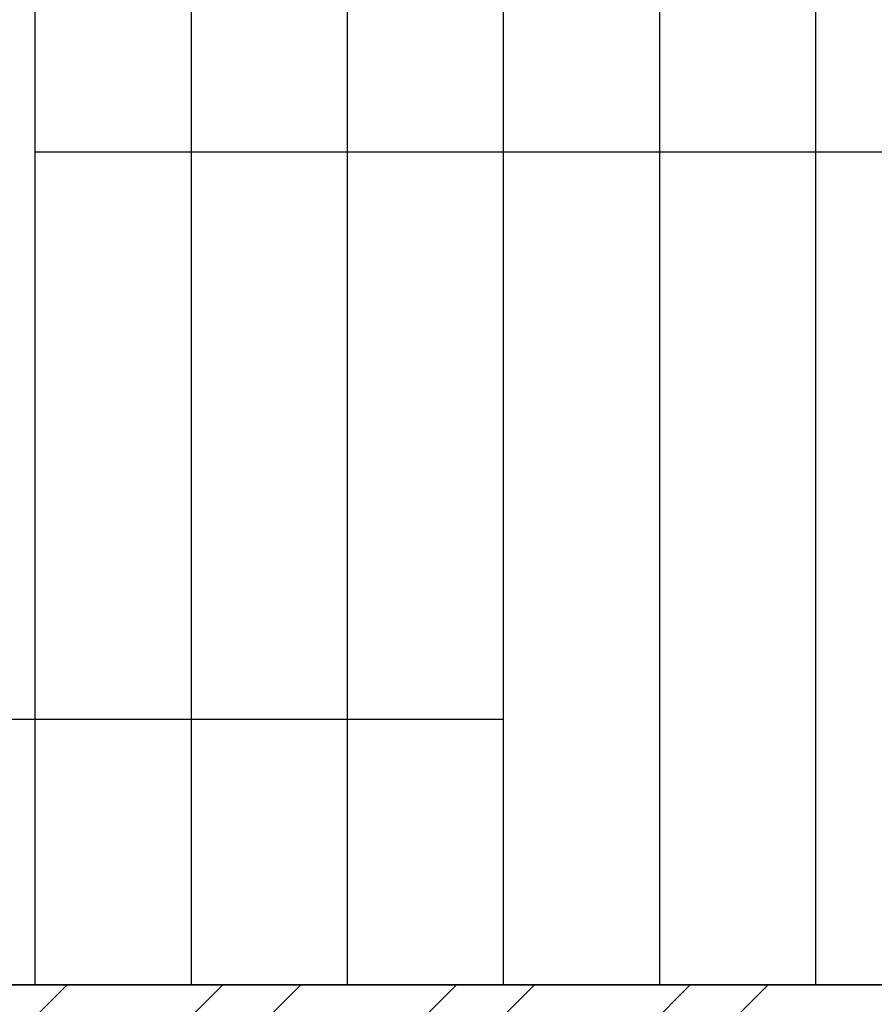
# Model space of a CAD drawing. Units: inches. Extents: x 1962 to 2771, y 1245 to 2660.
# Tile 34 of 114: x 2110 to 2159, y 1932 to 1989. Entities that reach past the tile are written whole.
import ezdxf

# ---------------------------------------------------------------- set-up
doc = ezdxf.new("R2010")
doc.units = ezdxf.units.IN
for name, color, linetype, lineweight in [('A-FLOR-STRS', 7, 'Continuous', 25), ('A-WALL', 7, 'Continuous', 35), ('A-WALL-PATT', 252, 'Continuous', 13)]:
    doc.layers.add(name, color=color, linetype=linetype, lineweight=lineweight)

msp = doc.modelspace()

# ---------------------------------------------------------------- hatches: boundary and pattern name
at = {"layer": 'A-WALL-PATT'}
h = msp.add_hatch(dxfattribs=at)
h.set_pattern_fill('ANSI32', color=256)
h.paths.add_polyline_path([(2090.8074, 2467.3437), (2141.6481, 2467.3437), (2141.6481, 2469.5937), (2141.6481, 2471.8437), (2086.3074, 2471.8437), (2086.3074, 2422.5333), (2090.8074, 2422.5333)])
h.paths.add_polyline_path([(2282.7664, 2471.8437), (2204.8982, 2471.8437), (2204.8982, 2467.3437), (2234.8074, 2467.3437), (2234.8074, 2311.3437), (2228.7492, 2311.3437), (2228.7492, 2306.8437), (2234.8074, 2306.8437), (2331.9227, 2306.8437), (2331.9227, 2309.0937), (2331.9227, 2311.3437), (2239.3074, 2311.3437), (2239.3074, 2467.3437), (2282.7664, 2467.3437), (2282.7664, 2469.5937)])
h.paths.add_polyline_path([(2471.4531, 2519.8437), (2552.011, 2519.8437), (2564.3996, 2519.8437), (2564.3996, 2511.1389), (2568.8996, 2511.1389), (2568.8996, 2524.3437), (2466.9531, 2524.3437), (2466.9531, 2471.8437), (2450.0749, 2471.8437), (2446.4672, 2471.8437), (2446.4672, 2467.3437), (2450.0749, 2467.3437), (2475.9988, 2467.3437), (2475.9988, 2469.5937), (2475.9988, 2471.8437), (2471.4531, 2471.8437)])
h.paths.add_polyline_path([(2575.2231, 2469.5937), (2575.2231, 2471.8437), (2568.8996, 2471.8437), (2568.8996, 2487.1389), (2564.3996, 2487.1389), (2564.3996, 2471.8437), (2556.511, 2471.8437), (2499.2904, 2471.8437), (2499.2904, 2467.3437), (2507.8074, 2467.3437), (2507.8074, 2311.3437), (2414.863, 2311.3437), (2414.863, 2306.8437), (2512.3074, 2306.8437), (2517.0114, 2306.8437), (2517.0114, 2309.0937), (2517.0114, 2311.3437), (2512.3074, 2311.3437), (2512.3074, 2467.3437), (2575.2231, 2467.3437)])
h.paths.add_polyline_path([(2660.8074, 2471.8437), (2600.9602, 2471.8437), (2600.9602, 2467.3437), (2656.3074, 2467.3437), (2656.3074, 2432.5704), (2660.8074, 2432.5704)])
h.paths.add_polyline_path([(2660.8074, 2372.5704), (2656.3074, 2372.5704), (2656.3074, 2311.3437), (2600.276, 2311.3437), (2600.276, 2309.0937), (2600.276, 2306.8437), (2656.3074, 2306.8437), (2656.3074, 2296.2593), (2660.8074, 2296.2593)])
h.paths.add_polyline_path([(2572.3074, 2306.8437), (2577.1385, 2306.8437), (2577.1385, 2311.3437), (2551.082, 2311.3437), (2551.082, 2306.8437), (2567.8074, 2306.8437), (2567.8074, 2258.8437), (2540.0574, 2258.8437), (2540.0574, 2256.5937), (2540.0574, 2254.3437), (2567.8074, 2254.3437), (2656.3074, 2254.3437), (2656.3074, 2236.9085), (2660.8074, 2236.9085), (2660.8074, 2272.2593), (2656.3074, 2272.2593), (2656.3074, 2258.8437), (2572.3074, 2258.8437)])
h.paths.add_polyline_path([(2512.3074, 2254.3437), (2518.8716, 2254.3437), (2518.8716, 2256.5937), (2518.8716, 2258.8437), (2507.8074, 2258.8437), (2507.8074, 2177.8437), (2567.8074, 2177.8437), (2567.8074, 2172.9628), (2572.3074, 2172.9628), (2572.3074, 2177.8437), (2656.3074, 2177.8437), (2656.3074, 2166.4846), (2660.8074, 2166.4846), (2660.8074, 2200.9085), (2656.3074, 2200.9085), (2656.3074, 2182.3437), (2512.3074, 2182.3437)])
h.paths.add_polyline_path([(2656.3074, 2129.8437), (2572.3074, 2129.8437), (2572.3074, 2150.3044), (2570.0574, 2150.3044), (2567.8074, 2150.3044), (2567.8074, 2129.8437), (2507.8074, 2129.8437), (2507.8074, 2116.3027), (2510.0574, 2116.3027), (2512.3074, 2116.3027), (2512.3074, 2125.3437), (2567.8074, 2125.3437), (2572.3074, 2125.3437), (2656.3074, 2125.3437)])
h.paths.add_polyline_path([(2090.8074, 2362.5333), (2086.3074, 2362.5333), (2086.3074, 2298.6242), (2090.8074, 2298.6242), (2090.8074, 2306.8437), (2174.8074, 2306.8437), (2174.8074, 2286.4178), (2179.3074, 2286.4178), (2179.3074, 2306.8437), (2192.8641, 2306.8437), (2192.8641, 2309.0937), (2192.8641, 2311.3437), (2090.8074, 2311.3437)])
h.paths.add_polyline_path([(2209.156, 2258.8437), (2179.3074, 2258.8437), (2179.3074, 2263.2236), (2177.0574, 2263.2236), (2174.8074, 2263.2236), (2174.8074, 2258.8437), (2090.8074, 2258.8437), (2090.8074, 2274.6242), (2086.3074, 2274.6242), (2086.3074, 2238.2967), (2088.5574, 2238.2967), (2090.8074, 2238.2967), (2090.8074, 2254.3437), (2209.156, 2254.3437)])
h.paths.add_polyline_path([(2090.8074, 2177.8437), (2234.8074, 2177.8437), (2234.8074, 2173.1428), (2239.3074, 2173.1428), (2239.3074, 2258.8437), (2230.8442, 2258.8437), (2230.8442, 2256.5937), (2230.8442, 2254.3437), (2234.8074, 2254.3437), (2234.8074, 2182.3437), (2090.8074, 2182.3437), (2090.8074, 2202.2967), (2086.3074, 2202.2967), (2086.3074, 2140.0389), (2090.8074, 2140.0389)])
h.paths.add_polyline_path([(2090.8074, 2080.0389), (2086.3074, 2080.0389), (2086.3074, 2033.8437), (2090.8074, 2033.8437)], flags=17)
h.paths.add_polyline_path([(2244.9405, 2033.8437), (2239.3074, 2033.8437), (2239.3074, 2142.0665), (2237.2592, 2142.0665), (2234.8074, 2142.0665), (2234.8074, 2033.8437), (2090.8074, 2033.8437), (2076.5204, 2033.8437), (2072.0204, 2033.8437), (2072.0204, 2000.4493), (2076.5204, 2000.4493), (2076.5204, 2029.3437), (2090.8074, 2029.3437), (2244.9405, 2029.3437), (2244.9405, 2031.5937)])
h.paths.add_polyline_path([(2234.8074, 1933.3437), (2076.5204, 1933.3437), (2076.5204, 1952.4493), (2074.2704, 1952.4493), (2072.0204, 1952.4493), (2072.0204, 1933.3437), (2072.0204, 1928.8437), (2234.8074, 1928.8437)])
h.paths.add_polyline_path([(2090.8074, 1928.8437), (2086.3074, 1928.8437), (2086.3074, 1906.5013), (2090.8074, 1906.5013)])
h.paths.add_polyline_path([(2090.8074, 1846.5013), (2086.3074, 1846.5013), (2086.3074, 1769.9917), (2088.5574, 1769.9917), (2090.8074, 1769.9917), (2090.8074, 1780.3437), (2234.8074, 1780.3437), (2234.8074, 1708.3437), (2230.3764, 1708.3437), (2230.3764, 1703.8437), (2239.3074, 1703.8437), (2239.3074, 1792.6669), (2237.0574, 1792.6669), (2234.8074, 1792.6669), (2234.8074, 1784.8437), (2090.8074, 1784.8437)])
h.paths.add_polyline_path([(2239.3074, 1928.8437), (2244.9405, 1928.8437), (2244.9405, 1931.0937), (2244.9405, 1933.3437), (2234.8074, 1933.3437), (2234.8074, 1928.8437), (2234.8074, 1825.5949), (2239.3074, 1825.5949)])
h.paths.add_polyline_path([(2148.0425, 1649.0937), (2148.0425, 1651.3437), (2090.8074, 1651.3437), (2090.8074, 1646.8437), (2148.0425, 1646.8437)], flags=0)
h.paths.add_polyline_path([(2207.5601, 1708.3437), (2090.8074, 1708.3437), (2090.8074, 1703.8437), (2174.8074, 1703.8437), (2174.8074, 1651.3437), (2170.4457, 1651.3437), (2170.4457, 1646.8437), (2195.9924, 1646.8437), (2195.9924, 1649.0937), (2195.9924, 1651.3437), (2179.3074, 1651.3437), (2179.3074, 1703.8437), (2207.5601, 1703.8437), (2207.5601, 1706.0937)])
h.paths.add_polyline_path([(2090.8074, 1733.9917), (2086.3074, 1733.9917), (2086.3074, 1696.1032), (2088.5574, 1696.1032), (2090.8074, 1696.1032)])
h.paths.add_polyline_path([(2090.8074, 1672.1032), (2086.3074, 1672.1032), (2086.3074, 1600.3335), (2090.8074, 1600.3335)])
h.paths.add_polyline_path([(2090.8074, 1540.3335), (2086.3074, 1540.3335), (2086.3074, 1486.3437), (2139.6766, 1486.3437), (2139.6766, 1490.8437), (2090.8074, 1490.8437)])
h.paths.add_polyline_path([(2302.3876, 1490.8437), (2239.3074, 1490.8437), (2239.3074, 1646.8437), (2335.9994, 1646.8437), (2335.9994, 1651.3437), (2229.884, 1651.3437), (2229.884, 1646.8437), (2234.8074, 1646.8437), (2234.8074, 1490.8437), (2202.7103, 1490.8437), (2202.7103, 1488.5937), (2202.7103, 1486.3437), (2275.0699, 1486.3437), (2275.0699, 1475.772), (2279.5699, 1475.772), (2279.5699, 1486.3437), (2302.3876, 1486.3437)])
h.paths.add_polyline_path([(2279.5699, 1451.772), (2275.0699, 1451.772), (2275.0699, 1438.3437), (2174.8074, 1438.3437), (2174.8074, 1486.3437), (2179.7922, 1486.3437), (2179.7922, 1490.8437), (2163.3585, 1490.8437), (2163.3585, 1488.5937), (2163.3585, 1486.3437), (2170.3074, 1486.3437), (2170.3074, 1433.8437), (2279.5699, 1433.8437)])
h.paths.add_polyline_path([(2427.2363, 1490.8437), (2375.8074, 1490.8437), (2375.8074, 1646.8437), (2381.6401, 1646.8437), (2381.6401, 1651.3437), (2365.887, 1651.3437), (2365.887, 1649.0937), (2365.887, 1646.8437), (2371.3074, 1646.8437), (2371.3074, 1490.8437), (2327.5627, 1490.8437), (2327.5627, 1488.5937), (2327.5627, 1486.3437), (2371.3074, 1486.3437), (2371.3074, 1433.8437), (2375.8074, 1433.8437), (2375.8074, 1486.3437), (2427.2363, 1486.3437)])
h.paths.add_polyline_path([(2512.3074, 1646.8437), (2519.4351, 1646.8437), (2519.4351, 1649.0937), (2519.4351, 1651.3437), (2507.8074, 1651.3437), (2416.0063, 1651.3437), (2416.0063, 1649.0937), (2416.0063, 1646.8437), (2507.8074, 1646.8437), (2507.8074, 1490.8437), (2497.0532, 1490.8437), (2497.0532, 1488.5937), (2497.0532, 1486.3437), (2574.9344, 1486.3437), (2574.9344, 1476.0181), (2579.4344, 1476.0181), (2579.4344, 1486.3437), (2584.4872, 1486.3437), (2584.3074, 1490.8437), (2512.3074, 1490.8437)])
h.paths.add_polyline_path([(2470.5091, 1486.3437), (2473.9767, 1486.3437), (2473.9767, 1490.8437), (2449.6605, 1490.8437), (2449.6605, 1488.5937), (2449.6605, 1486.3437), (2466.0091, 1486.3437), (2466.0091, 1433.8437), (2470.5091, 1433.8437), (2579.4344, 1433.8437), (2579.4344, 1452.0181), (2574.9344, 1452.0181), (2574.9344, 1438.3437), (2554.5091, 1438.3437), (2470.5091, 1438.3437)])
h.paths.add_polyline_path([(2656.3074, 1490.8437), (2611.86, 1490.8437), (2611.86, 1486.3437), (2656.3074, 1486.3437)])
h.paths.add_polyline_path([(2660.8074, 1532.7007), (2658.5574, 1532.7007), (2656.3074, 1532.7007), (2656.3074, 1486.3437), (2660.8074, 1486.3437)])
h.paths.add_polyline_path([(2660.8074, 1664.9663), (2656.3074, 1664.9663), (2656.3074, 1651.3437), (2602.2313, 1651.3437), (2602.2313, 1646.8437), (2656.3074, 1646.8437), (2656.3074, 1592.7007), (2660.8074, 1592.7007)])
h.paths.add_polyline_path([(2660.8074, 1724.5221), (2656.3074, 1724.5221), (2656.3074, 1703.8437), (2542.4725, 1703.8437), (2542.4725, 1699.3437), (2567.8074, 1699.3437), (2567.8074, 1651.3437), (2552.7766, 1651.3437), (2552.7766, 1649.0937), (2552.7766, 1646.8437), (2577.2878, 1646.8437), (2577.2878, 1649.0937), (2577.2878, 1651.3437), (2572.3074, 1651.3437), (2572.3074, 1699.3437), (2656.3074, 1699.3437), (2656.3074, 1688.9663), (2660.8074, 1688.9663)])
h.paths.add_polyline_path([(2660.8074, 1880.6524), (2656.3074, 1880.6524), (2656.3074, 1832.8437), (2512.3074, 1832.8437), (2512.3074, 1837.8959), (2507.8074, 1837.8959), (2507.8074, 1828.3437), (2567.8074, 1828.3437), (2567.8074, 1804.3437), (2572.3074, 1804.3437), (2572.3074, 1828.3437), (2656.3074, 1828.3437), (2656.3074, 1818.6778), (2660.8074, 1818.6778)])
h.paths.add_polyline_path([(2660.8074, 1794.6778), (2656.3074, 1794.6778), (2656.3074, 1780.3437), (2572.3074, 1780.3437), (2572.3074, 1783.0303), (2570.0574, 1783.0303), (2567.8074, 1783.0303), (2567.8074, 1780.3437), (2507.8074, 1780.3437), (2507.8074, 1699.3437), (2517.8858, 1699.3437), (2517.8858, 1701.5937), (2517.8858, 1703.8437), (2512.3074, 1703.8437), (2512.3074, 1775.8437), (2656.3074, 1775.8437), (2656.3074, 1760.5221), (2660.8074, 1760.5221)])
h.paths.add_polyline_path([(2660.8074, 1981.3437), (2660.8074, 2020.2808), (2658.5574, 2020.2808), (2656.3074, 2020.2808), (2656.3074, 1981.3437), (2512.3074, 1981.3437), (2512.3074, 2086.6996), (2507.8074, 2086.6996), (2507.8074, 1981.3437), (2375.8074, 1981.3437), (2375.8074, 1986.8505), (2373.5574, 1986.8505), (2371.3074, 1986.8505), (2371.3074, 1973.2607), (2375.8074, 1973.2607), (2375.8074, 1976.8437), (2507.8074, 1976.8437), (2507.8074, 1865.4281), (2510.0574, 1865.4281), (2512.3074, 1865.4281), (2512.3074, 1976.8437), (2660.8074, 1976.8437)])
h.paths.add_polyline_path([(2375.8074, 1940.297), (2373.5574, 1940.297), (2371.3074, 1940.297), (2371.3074, 1933.3437), (2278.4434, 1933.3437), (2278.4434, 1928.8437), (2371.3074, 1928.8437), (2371.3074, 1651.3437), (2375.8074, 1651.3437)])
h.paths.add_polyline_path([(2660.8074, 1976.8437), (2656.3074, 1976.8437), (2656.3074, 1940.6524), (2660.8074, 1940.6524)], flags=17)
h.paths.add_polyline_path([(2660.8074, 2142.4846), (2656.3074, 2142.4846), (2656.3074, 2080.2808), (2660.8074, 2080.2808)])
h.paths.add_polyline_path([(2381.4189, 2311.3437), (2375.8074, 2311.3437), (2375.8074, 2467.3437), (2424.7242, 2467.3437), (2424.7242, 2469.5937), (2424.7242, 2471.8437), (2375.8074, 2471.8437), (2375.8074, 2524.3437), (2371.3074, 2524.3437), (2371.3074, 2471.8437), (2307.2097, 2471.8437), (2307.2097, 2467.3437), (2371.3074, 2467.3437), (2371.3074, 2311.3437), (2366.8901, 2311.3437), (2366.8901, 2306.8437), (2371.3074, 2306.8437), (2371.3074, 2033.8437), (2279.6589, 2033.8437), (2279.6589, 2029.3437), (2371.3074, 2029.3437), (2371.3074, 2014.2598), (2375.8074, 2014.2598), (2375.8074, 2306.8437), (2381.4189, 2306.8437)])
h.paths.add_polyline_path([(2263.3074, 2524.3437), (2170.3074, 2524.3437), (2170.3074, 2519.8437), (2170.3074, 2471.8437), (2165.0312, 2471.8437), (2165.0312, 2467.3437), (2179.6721, 2467.3437), (2179.6721, 2469.5161), (2179.6721, 2471.8437), (2174.8074, 2471.8437), (2174.8074, 2519.8437), (2258.8074, 2519.8437), (2258.8074, 2511.6436), (2263.3074, 2511.6436)])
h.paths.add_polyline_path([(2245.0232, 1361.4123), (2492.9468, 1361.4123), (2492.9468, 1398.505), (2245.0232, 1398.505)], flags=9)
h.paths.add_polyline_path([(2388.1434, 2086.6936), (2425.0704, 2086.6936), (2425.0704, 2105.3509), (2388.1434, 2105.3509)], flags=9)
h.paths.add_polyline_path([(2404.922, 2242.6744), (2445.7337, 2242.6744), (2445.7337, 2261.3318), (2404.922, 2261.3318)], flags=9)
h.paths.add_polyline_path([(2269.4107, 2156.7935), (2306.3378, 2156.7935), (2306.3378, 2175.4508), (2269.4107, 2175.4508)], flags=9)
h.paths.add_polyline_path([(2269.3277, 2233.4343), (2306.2547, 2233.4343), (2306.2547, 2252.0917), (2269.3277, 2252.0917)], flags=9)
h.paths.add_polyline_path([(2431.6052, 2320.6922), (2470.4456, 2320.6922), (2470.4456, 2339.3495), (2431.6052, 2339.3495)], flags=25)
h.paths.add_polyline_path([(2249.6902, 2315.7608), (2288.5306, 2315.7608), (2288.5306, 2334.4182), (2249.6902, 2334.4182)], flags=25)
h.paths.add_polyline_path([(2096.9301, 2314.3181), (2135.7704, 2314.3181), (2135.7704, 2332.9755), (2096.9301, 2332.9755)], flags=25)
h.paths.add_polyline_path([(2134.3475, 2285.7089), (2161.4655, 2285.7089), (2161.4655, 2304.3662), (2134.3475, 2304.3662)], flags=9)
h.paths.add_polyline_path([(2126.5155, 2209.4076), (2159.9227, 2209.4076), (2159.9227, 2228.065), (2126.5155, 2228.065)], flags=25)
h.paths.add_polyline_path([(2110.5753, 2141.5299), (2149.4157, 2141.5299), (2149.4157, 2160.1872), (2110.5753, 2160.1872)], flags=25)
h.paths.add_polyline_path([(2249.8618, 1968.3317), (2286.3966, 1968.3317), (2286.3966, 1986.989), (2249.8618, 1986.989)], flags=9)
h.paths.add_polyline_path([(2395.9507, 1777.0051), (2436.7624, 1777.0051), (2436.7624, 1795.6625), (2395.9507, 1795.6625)], flags=9)
h.paths.add_polyline_path([(2398.5259, 1888.5651), (2435.0062, 1888.5651), (2435.0062, 1907.2224), (2398.5259, 1907.2224)], flags=25)
h.paths.add_polyline_path([(2259.3506, 1728.3559), (2296.2776, 1728.3559), (2296.2776, 1747.0132), (2259.3506, 1747.0132)], flags=9)
h.paths.add_polyline_path([(2271.3698, 1845.268), (2308.2968, 1845.268), (2308.2968, 1863.9253), (2271.3698, 1863.9253)], flags=9)
h.paths.add_polyline_path([(2120.9355, 1786.3027), (2159.7759, 1786.3027), (2159.7759, 1804.9601), (2120.9355, 1804.9601)], flags=25)
h.paths.add_polyline_path([(2121.3164, 1732.1043), (2154.7236, 1732.1043), (2154.7236, 1750.7616), (2121.3164, 1750.7616)], flags=25)
h.paths.add_polyline_path([(2118.3706, 1678.8997), (2147.5282, 1678.8997), (2147.5282, 1697.557), (2118.3706, 1697.557)], flags=25)
h.paths.add_polyline_path([(2385.9227, 1493.557), (2424.763, 1493.557), (2424.763, 1512.2143), (2385.9227, 1512.2143)], flags=25)
h.paths.add_polyline_path([(2248.7058, 1500.0256), (2287.5462, 1500.0256), (2287.5462, 1518.6829), (2248.7058, 1518.6829)], flags=25)
h.paths.add_polyline_path([(2104.1669, 1617.3771), (2143.0073, 1617.3771), (2143.0073, 1636.0344), (2104.1669, 1636.0344)], flags=9)
h.paths.add_polyline_path([(2096.0714, 1447.8824), (2137.3845, 1447.8824), (2137.3845, 1458.1859), (2096.0714, 1458.1859)], flags=9)
h.paths.add_polyline_path([(2180.6114, 1440.325), (2209.7689, 1440.325), (2209.7689, 1458.9823), (2180.6114, 1458.9823)], flags=25)
h.paths.add_polyline_path([(2316.1698, 1447.9637), (2357.4829, 1447.9637), (2357.4829, 1458.2673), (2316.1698, 1458.2673)], flags=9)
h.paths.add_polyline_path([(2397.6187, 1447.9637), (2438.9318, 1447.9637), (2438.9318, 1458.2673), (2397.6187, 1458.2673)], flags=9)
h.paths.add_polyline_path([(2473.0778, 1439.5953), (2502.2354, 1439.5953), (2502.2354, 1458.2527), (2473.0778, 1458.2527)], flags=25)
h.paths.add_polyline_path([(2589.7027, 1447.8819), (2631.0158, 1447.8819), (2631.0158, 1458.1855), (2589.7027, 1458.1855)], flags=9)
h.paths.add_polyline_path([(2522.4009, 1497.5285), (2561.2413, 1497.5285), (2561.2413, 1516.1859), (2522.4009, 1516.1859)], flags=25)
h.paths.add_polyline_path([(2579.6565, 1671.3482), (2608.8141, 1671.3482), (2608.8141, 1690.0056), (2579.6565, 1690.0056)], flags=25)
h.paths.add_polyline_path([(2544.7038, 1725.5064), (2578.1111, 1725.5064), (2578.1111, 1744.1637), (2544.7038, 1744.1637)], flags=25)
h.paths.add_polyline_path([(2578.1191, 1807.472), (2607.2766, 1807.472), (2607.2766, 1826.1293), (2578.1191, 1826.1293)], flags=25)
h.paths.add_polyline_path([(2595.0614, 1835.1839), (2633.9018, 1835.1839), (2633.9018, 1853.8413), (2595.0614, 1853.8413)], flags=25)
h.paths.add_polyline_path([(2567.0097, 2097.7035), (2605.8501, 2097.7035), (2605.8501, 2116.3609), (2567.0097, 2116.3609)], flags=9)
h.paths.add_polyline_path([(2586.644, 2134.6454), (2615.8015, 2134.6454), (2615.8015, 2153.3027), (2586.644, 2153.3027)], flags=9)
h.paths.add_polyline_path([(2544.6185, 2212.6783), (2578.0258, 2212.6783), (2578.0258, 2231.3356), (2544.6185, 2231.3356)], flags=25)
h.paths.add_polyline_path([(2577.0273, 2256.9023), (2606.1849, 2256.9023), (2606.1849, 2275.5597), (2577.0273, 2275.5597)], flags=24)
h.paths.add_polyline_path([(2605.2683, 2315.2821), (2644.1087, 2315.2821), (2644.1087, 2333.9395), (2605.2683, 2333.9395)], flags=25)
h.paths.add_polyline_path([(2583.1244, 2496.1815), (2624.4375, 2496.1815), (2624.4375, 2506.4851), (2583.1244, 2506.4851)], flags=9)
h.paths.add_polyline_path([(2474.761, 2497.0823), (2503.9185, 2497.0823), (2503.9185, 2515.7397), (2474.761, 2515.7397)], flags=25)
h.paths.add_polyline_path([(2387.5787, 2494.2563), (2428.902, 2494.2563), (2428.902, 2504.5598), (2387.5787, 2504.5598)], flags=9)
h.paths.add_polyline_path([(2300.1657, 2500.1564), (2341.4788, 2500.1564), (2341.4788, 2510.46), (2300.1657, 2510.46)], flags=25)
h.paths.add_polyline_path([(2176.8589, 2497.5843), (2206.0165, 2497.5843), (2206.0165, 2516.2416), (2176.8589, 2516.2416)], flags=25)
h.paths.add_polyline_path([(2097.4668, 2494.9762), (2138.7799, 2494.9762), (2138.7799, 2505.2798), (2097.4668, 2505.2798)], flags=9)

# ---------------------------------------------------------------- linework, layer by layer
at = {"layer": 'A-FLOR-STRS'}
for p, q in [((2111.0955, 2029.3437), (2111.0955, 1933.3437)), ((2120.0955, 2029.3437), (2120.0955, 1933.3437)), ((2129.0955, 2029.3437), (2129.0955, 1933.3437)), ((2138.0955, 2029.3437), (2138.0955, 1933.3437)), ((2147.0955, 2029.3437), (2147.0955, 1933.3437)), ((2156.0955, 2029.3437), (2156.0955, 1933.3437)), ((2111.0955, 1981.3437), (2228.0955, 1981.3437)), ((2096.9843, 1948.6514), (2138.0955, 1948.6514))]:
    msp.add_line(p, q, dxfattribs=at)
at = {"layer": 'A-WALL'}
msp.add_line((2076.5204, 1933.3437), (2244.9405, 1933.3437), dxfattribs=at)

doc.saveas('drawing.dxf')
